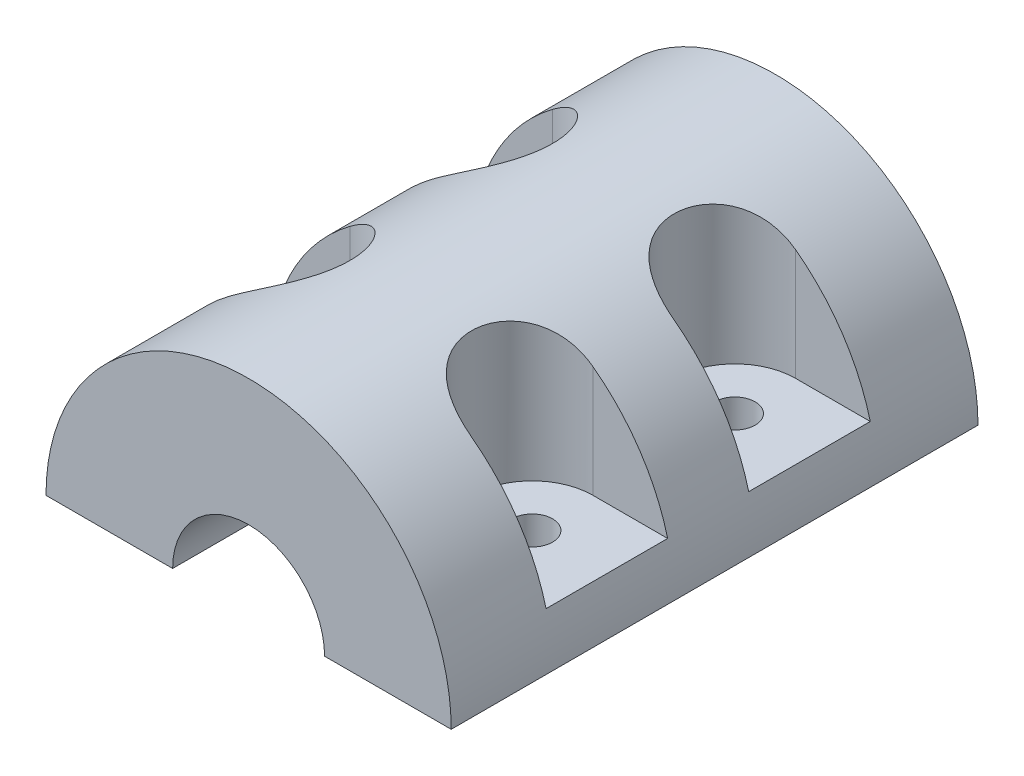
from build123d import *

# Parameters (mm, degrees)
BLOCK_BODY_260_DEPTH                   = 130
BOLT_START                             = 25
BOLT_POCKET_60X80_DEPTH                = 260
BOLT_POCKET_MIRROR_RIGHT_COPY_1_DEPTH  = 260
BOLT_HOLE_SKETCH_R                     = 10
BOLT_HOLE_CUT_DEPTH                    = 260
BOLT_HOLE_MIRROR_RIGHT_COPY_1_SKETCH_R = 10
BOLT_HOLE_MIRROR_RIGHT_COPY_1_DEPTH    = 260


with BuildPart() as part:
    # Block Profile Sketch → Block Body 260 (new, symmetric)
    with BuildSketch(Plane.XY):
        with BuildLine():
            Line((-100, 0), (-37.5, 0))
            ThreePointArc((-37.5, 0), (0, 37.5), (37.5, 0))
            Line((37.5, 0), (100, 0))
            ThreePointArc((100, 0), (0, 100), (-100, 0))
        make_face()
    extrude(amount=BLOCK_BODY_260_DEPTH, both=True)

    # Bolt Pocket Sketch → Bolt Pocket 60x80 (cut)
    with BuildSketch(Plane(origin=(0, 0, 0), x_dir=(1, 0, 0), z_dir=(0, 1, 0)).offset(BOLT_START)):
        with BuildLine():
            Line((-60, -20), (-100, -20))
            Line((-100, -20), (-100, -80))
            Line((-100, -80), (-60, -80))
            ThreePointArc((-60, -80), (-30, -50), (-60, -20))
        make_face()
    bolt_pocket_60x80 = extrude(amount=BOLT_POCKET_60X80_DEPTH, mode=Mode.SUBTRACT)

    # Bolt Pocket Mirror Front: Bolt Pocket 60x80 across plane
    add(bolt_pocket_60x80.mirror(Plane.XY), mode=Mode.SUBTRACT)

    # Bolt Pocket Mirror Right: Bolt Pocket 60x80 across plane
    add(bolt_pocket_60x80.mirror(Plane(origin=(0, 0, 0), x_dir=(0, 0, 1), z_dir=(1, 0, 0))), mode=Mode.SUBTRACT)

    # Bolt Pocket Mirror Right copy 1 sketch → Bolt Pocket Mirror Right copy 1 (cut)
    with BuildSketch(Plane(origin=(0, 0, 0), x_dir=(-1, 0, 0), z_dir=(0, 1, 0)).offset(BOLT_START)):
        with BuildLine():
            Line((-60, -20), (-100, -20))
            Line((-100, -20), (-100, -80))
            Line((-100, -80), (-60, -80))
            ThreePointArc((-60, -80), (-30, -50), (-60, -20))
        make_face()
    extrude(amount=BOLT_POCKET_MIRROR_RIGHT_COPY_1_DEPTH, mode=Mode.SUBTRACT)

    # Bolt Hole Sketch → Bolt Hole Cut (cut)
    with BuildSketch(Plane(origin=(0, 25, 0), x_dir=(1, 0, 0), z_dir=(0, 1, 0))):
        with Locations(Location((-60, -50, 0), (0, 0, 270))):
            Circle(BOLT_HOLE_SKETCH_R)
    bolt_hole_cut = extrude(amount=-BOLT_HOLE_CUT_DEPTH, mode=Mode.SUBTRACT)

    # Bolt Hole Mirror Front: Bolt Hole Cut across plane
    add(bolt_hole_cut.mirror(Plane.XY), mode=Mode.SUBTRACT)

    # Bolt Hole Mirror Right: Bolt Hole Cut across plane
    add(bolt_hole_cut.mirror(Plane(origin=(0, 0, 0), x_dir=(0, 0, 1), z_dir=(1, 0, 0))), mode=Mode.SUBTRACT)

    # Bolt Hole Mirror Right copy 1 sketch → Bolt Hole Mirror Right copy 1 (cut)
    with BuildSketch(Plane(origin=(0, 25, 0), x_dir=(-1, 0, 0), z_dir=(0, 1, 0))):
        with Locations(Location((-60, -50, 0), (0, 0, 270))):
            Circle(BOLT_HOLE_MIRROR_RIGHT_COPY_1_SKETCH_R)
    extrude(amount=-BOLT_HOLE_MIRROR_RIGHT_COPY_1_DEPTH, mode=Mode.SUBTRACT)


solid = part.part
